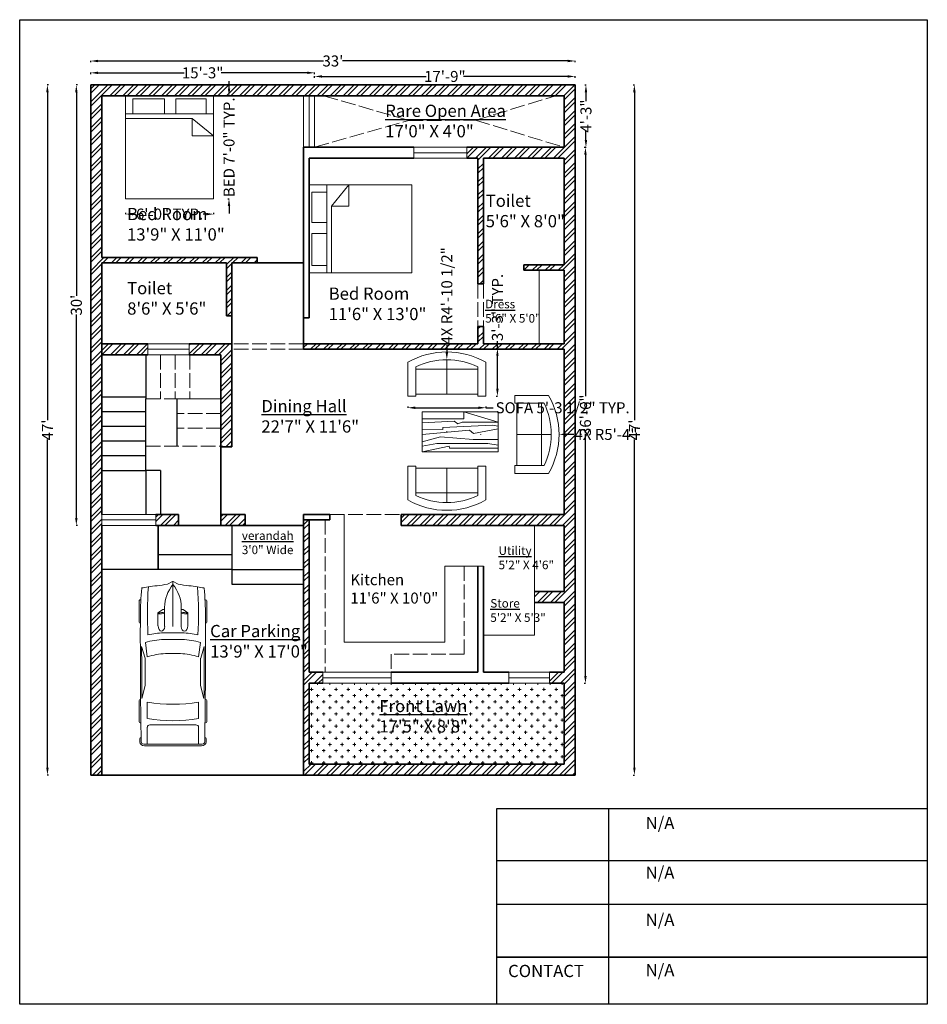
# Model space of a CAD drawing. Units: inches. Extents: x -42 to 700, y -732 to 72.
import ezdxf

# ---------------------------------------------------------------- set-up
doc = ezdxf.new("R2010")
doc.units = ezdxf.units.IN
doc.header["$MEASUREMENT"] = 0
doc.linetypes.add('ACAD_ISO02W100', pattern=[15, 12, -3])
for name, color, linetype, lineweight in [('A-ANNO-DIMS', 2, 'Continuous', 18), ('A-ANNO-TEXT', 7, 'Continuous', 18), ('A-ANNO-TTLB', 7, 'Continuous', 25), ('A-AREA-IDEN', 7, 'Continuous', 25), ('A-EQPM-VEHI', 8, 'Continuous', 18), ('A-FLOR-CASE', 8, 'Continuous', 18), ('A-FLOR-CASE-HIDN', 8, 'ACAD_ISO02W100', 13), ('A-FLOR-OPEN', 9, 'ACAD_ISO02W100', 13), ('A-FLOR-STRS', 6, 'Continuous', 25), ('A-FLOR-STRS-OVHD', 6, 'ACAD_ISO02W100', 18), ('A-FURN', 8, 'Continuous', 18), ('A-GLAZ', 5, 'Continuous', 18), ('A-WALL', 7, 'Continuous', 35), ('A-WALL-OVHD', 7, 'ACAD_ISO02W100', 18), ('A-WALL-PATT', 252, 'Continuous', 13), ('L-PLNT-PATT', 3, 'Continuous', 13)]:
    doc.layers.add(name, color=color, linetype=linetype, lineweight=lineweight)
doc.styles.get("Standard").update_dxf_attribs({"font": 'arial.ttf'})
doc.dimstyles.get("Standard").update_dxf_attribs({"dimtxt": 9, "dimasz": 6, "dimexe": 0.18, "dimexo": 0.0625, "dimgap": 0.09, "dimtad": 0, "dimdec": 0, "dimzin": 0, "dimdsep": 46, "dimlunit": 3, "dimtxsty": 'Standard', "dimcen": 0.09, "dimadec": 0, "dimazin": 0, "dimtfac": 1, "dimtdec": 0, "dimtofl": 0, "dimtmove": 0, "dimatfit": 3, "dimfxl": 1, "dimfxlon": 1, "dimtolj": 1, "dimtzin": 0, "dimarcsym": 0})

# ---------------------------------------------------------------- blocks, each defined once
blk = doc.blocks.new('A$C01575E38')
for p, q in [((0, 0), (0, 0.65)), ((0, 0), (0, 0.65)), ((0.75, 0.039), (0.75, 0.7)), ((0.75, 0.039), (0.75, 0.7)), ((1.5, 0.65), (1.5, 0)), ((1.5, 0.65), (1.5, 0)), ((0.15, 0), (0.15, 0.563)), ((0.15, 0), (0.15, 0.563)), ((0.15, 0.515), (1.35, 0.515)), ((0.15, 0.515), (1.35, 0.515)), ((1.35, 0), (1.35, 0.563)), ((1.35, 0), (1.35, 0.563)), ((0.15, 0), (0, 0)), ((0.15, 0), (0, 0)), ((0.15, 0.039), (1.35, 0.039)), ((0.15, 0.039), (1.35, 0.039)), ((1.5, 0), (1.35, 0)), ((1.5, 0), (1.35, 0))]:
    blk.add_line(p, q)
for centre, radius, start, end in [((0.75, -0.656), 1.506, 60.1372, 119.8628), ((0.75, -0.656), 1.506, 60.1372, 119.8628), ((0.75, -0.685), 1.385, 64.3208, 115.6792), ((0.75, -0.685), 1.385, 64.3208, 115.6792)]:
    blk.add_arc(centre, radius, start, end)
blk = doc.blocks.new('*U3')
for p, q in [((21.1, 37.4), (21.1, 36.8)), ((46.6, 38.9), (22.4, 38.9)), ((47.8, 37.4), (47.8, 37.4)), ((88, 31.9), (74.8, 35.9)), ((134.3, 35.6), (119.3, 31.8)), ((135.5, 37.1), (135.5, 37.4)), ((136.7, 38.9), (160.9, 38.9)), ((162.1, 37.4), (162.1, 36.8)), ((70, 31.5), (86.4, 29.4)), ((138.4, 29.4), (157.2, 29.4)), ((164.5, 26.4), (164.5, -26.4)), ((186.5, 29.4), (167, 29.4)), ((186.5, -33.5), (186.5, 33.5)), ((188.4, -32.8), (188.4, 32.8)), ((32.3, 11.6), (36.1, 17.2)), ((36.1, 17.2), (50.9, 17.2)), ((3.3, 6.1), (0.1, 0.4)), ((29.8, 9.5), (51.7, 9.5)), ((32.1, 9.5), (32.1, 11.2)), ((58.9, -10.8), (58.9, 10.8)), ((66.6, -10.5), (66.6, 10.5)), ((82.7, 8.5), (82.7, -8.5)), ((186.5, -10.5), (186.5, 10.5)), ((0, 0), (51.7, 0)), ((0.1, -0.4), (3.3, -6.1)), ((29.8, -9.5), (51.7, -9.5)), ((32.1, -9.5), (32.1, -11.2)), ((32.3, -11.6), (36.1, -17.2)), ((36.1, -17.2), (50.9, -17.2)), ((86.4, -29.4), (70, -31.5)), ((88, -31.9), (74.8, -35.9)), ((134.3, -35.6), (119.3, -31.8)), ((157.2, -29.4), (138.4, -29.4)), ((167, -29.4), (186.5, -29.4)), ((21.1, -37.4), (21.1, -36.8)), ((46.6, -38.9), (22.4, -38.9)), ((47.8, -37.4), (47.8, -37.4)), ((135.5, -37.1), (135.5, -37.4)), ((136.7, -38.9), (160.9, -38.9)), ((162.1, -37.4), (162.1, -36.8))]:
    blk.add_line(p, q)
for centre, major_axis, ratio, start_param, end_param in [((266, -27.5), (0, 313.3), 0.842304, 1.367076, 1.39176), ((41.2, -490.9), (0, 528.2), 0.842304, 0.00281, 0.075598), ((22.4, 37.4), (0, -1.48), 0.842304, 3.141593, 4.712389), ((64.5, -10555.6), (0, 10593), 0.842304, -0.013397, 0.002797), ((46.6, 37.4), (0, 1.48), 0.842304, -1.570796, 0), ((64.5, -10555.6), (0, -10591.5), 0.842304, 3.133765, 3.140441), ((136.7, 37.4), (0, -1.48), 0.842304, 3.141593, 4.712389), ((160.9, 37.4), (0, 1.48), 0.842304, -1.570796, 0), ((180.6, 35.8), (0, 2.22), 0.842304, -0.013017, 1.249894), ((64.5, -10556.4), (0, 10595.3), 0.842304, -0.013397, -0.013017), ((184, 32.8), (0, -5.25), 0.842304, 1.570796, 3.128196), ((184, 33.5), (0, -2.96), 0.842304, 1.570796, 3.128196), ((259.2, -27.5), (0, -305.3), 0.842304, 4.528606, 4.561838), ((37.5, -594), (0, -623.3), 0.842304, 3.096046, 3.200911), ((134.4, 5.4), (0, -89.8), 0.842304, 4.449482, 4.652344), ((135.3, 5.4), (0, 81.8), 0.842304, 1.245306, 1.50788), ((149.6, 2.8), (0, -79.6), 0.842304, 4.372215, 4.640744), ((95.8, -3666.4), (0, -3698.2), 0.842304, 3.134049, 3.144098), ((17.1, 0), (0, 147), 0.842304, 4.511394, 4.913384), ((35.9, 0), (0, 147), 0.842304, 4.511394, 4.913384), ((167, 26.4), (0, 2.96), 0.842304, 0, 1.570796), ((-204.5, 52.4), (0, -251), 0.842304, 1.385369, 1.434372), ((32.7, 11.2), (0, 0.74), 0.842304, 0.879714, 1.570796), ((13, 17), (0, 27.4), 0.842304, 4.435146, 4.718221), ((14.2, 17), (0, 27.4), 0.842304, 4.435146, 4.718221), ((50.8, 13.3), (6.34, -0.36), 0.603834, -1.395552, 1.581315), ((0.6, 0), (0, -0.74), 0.842304, 4.131459, 5.293319), ((29.8, -46.7), (0, 56.2), 0.842304, 0, 0.590319), ((-204.5, -52.4), (0, 251), 0.842304, -1.434372, -1.385369), ((29.8, 46.7), (0, 56.2), 0.842304, 2.551274, 3.141593), ((32.7, -11.2), (0, -0.74), 0.842304, 4.712389, 5.403472), ((13, -17), (0, -27.4), 0.842304, 1.564964, 1.848039), ((14.2, -17), (0, -27.4), 0.842304, 1.564964, 1.848039), ((134.4, -5.4), (0, -89.8), 0.842304, -1.510751, -1.307889), ((135.3, -5.4), (0, -81.8), 0.842304, -1.50788, -1.245306), ((149.6, -2.8), (0, -79.6), 0.842304, -1.499151, -1.230623), ((259.2, 27.5), (0, 305.3), 0.842304, 1.721348, 1.754579), ((266, 27.5), (0, 313.3), 0.842304, 1.749832, 1.774517), ((37.5, 594), (0, -623.3), 0.842304, -0.059319, 0.045547), ((95.8, 3666.4), (0, -3698.2), 0.842304, -0.002505, 0.007544), ((167, -26.4), (0, -2.96), 0.842304, 4.712389, 6.283185), ((184, -32.8), (0, -5.25), 0.842304, 0.013397, 1.570796), ((184, -33.5), (0, 2.96), 0.842304, 3.15499, 4.712389), ((41.2, 490.9), (0, -528.2), 0.842304, -0.075598, -0.00281), ((22.4, -37.4), (0, 1.48), 0.842304, 1.570796, 3.141593), ((64.5, 10555.6), (0, 10593), 0.842304, 3.138796, 3.15499), ((46.6, -37.4), (0, -1.48), 0.842304, 0, 1.570796), ((64.5, 10555.6), (0, -10591.5), 0.842304, 0.001152, 0.007828), ((136.7, -37.4), (0, -1.48), 0.842304, -1.570796, 0), ((160.9, -37.4), (0, 1.48), 0.842304, 3.141593, 4.712389), ((180.6, -35.8), (0, -2.22), 0.842304, -1.249894, 0.013017), ((64.5, 10556.4), (0, 10595.3), 0.842304, 3.15461, 3.15499)]:
    blk.add_ellipse(centre, major_axis=major_axis, ratio=ratio, start_param=start_param, end_param=end_param)
at = {"extrusion": (0, 0, -1)}
blk.add_ellipse((50.8, -13.3), major_axis=(6.34, 0.36), ratio=0.603834, start_param=-1.395552, end_param=1.581315, dxfattribs=at)
blk = doc.blocks.new('*D4')
at = {"layer": 'A-ANNO-DIMS', "color": 0, "lineweight": -2, "transparency": 16777216}
for p, q in [((15.72, 27.92), (15.72, 29.1)), ((21.72, 28.92), (92.09, 28.92)), ((192.72, 28.92), (122.34, 28.92)), ((198.72, 27.92), (198.72, 29.1))]:
    blk.add_line(p, q, dxfattribs=at)
at = {"layer": 'A-ANNO-DIMS', "color": 0, "transparency": 16777216}
for points in [[(21.72, 29.92), (21.72, 27.92), (15.72, 28.92)], [(192.72, 29.92), (192.72, 27.92), (198.72, 28.92)]]:
    blk.add_solid(points, dxfattribs=at)
at = {"layer": 'Defpoints', "color": 0, "transparency": 16777216}
for p in [(198.72, 28.92), (15.72, 19.05), (198.72, 19.05)]:
    blk.add_point(p, dxfattribs=at)
at = {"layer": 'A-ANNO-DIMS', "color": 0, "transparency": 16777216, "insert": (107.22, 28.92), "char_height": 9, "attachment_point": 5}
blk.add_mtext('\\A1;15\'-3"', dxfattribs=at)
blk = doc.blocks.new('*D5')
at = {"layer": 'A-ANNO-DIMS', "color": 0, "lineweight": -2, "transparency": 16777216}
for p, q in [((15.72, 37.59), (15.72, 38.77)), ((21.72, 38.59), (205.99, 38.59)), ((405.72, 38.59), (221.44, 38.59)), ((411.72, 37.59), (411.72, 38.77))]:
    blk.add_line(p, q, dxfattribs=at)
at = {"layer": 'A-ANNO-DIMS', "color": 0, "transparency": 16777216}
for points in [[(21.72, 39.59), (21.72, 37.59), (15.72, 38.59)], [(405.72, 39.59), (405.72, 37.59), (411.72, 38.59)]]:
    blk.add_solid(points, dxfattribs=at)
at = {"layer": 'Defpoints', "color": 0, "transparency": 16777216}
for p in [(411.72, 38.59), (15.72, 19.05), (411.72, 19.05)]:
    blk.add_point(p, dxfattribs=at)
at = {"layer": 'A-ANNO-DIMS', "color": 0, "transparency": 16777216, "insert": (213.72, 38.59), "char_height": 9, "attachment_point": 5}
blk.add_mtext("\\A1;33'", dxfattribs=at)
blk = doc.blocks.new('*D6')
at = {"layer": 'A-ANNO-DIMS', "color": 0, "lineweight": -2, "transparency": 16777216}
for p, q in [((198.72, 24.95), (198.72, 26.13)), ((204.72, 25.95), (290.09, 25.95)), ((405.72, 25.95), (320.34, 25.95)), ((411.72, 24.95), (411.72, 26.13))]:
    blk.add_line(p, q, dxfattribs=at)
at = {"layer": 'A-ANNO-DIMS', "color": 0, "transparency": 16777216}
for points in [[(204.72, 26.95), (204.72, 24.95), (198.72, 25.95)], [(405.72, 26.95), (405.72, 24.95), (411.72, 25.95)]]:
    blk.add_solid(points, dxfattribs=at)
at = {"layer": 'Defpoints', "color": 0, "transparency": 16777216}
for p in [(411.72, 25.95), (198.72, 19.05), (411.72, 19.05)]:
    blk.add_point(p, dxfattribs=at)
at = {"layer": 'A-ANNO-DIMS', "color": 0, "transparency": 16777216, "insert": (305.22, 25.95), "char_height": 9, "attachment_point": 5}
blk.add_mtext('\\A1;17\'-9"', dxfattribs=at)
blk = doc.blocks.new('*D7')
at = {"layer": 'A-ANNO-DIMS', "color": 0, "lineweight": -2, "transparency": 16777216}
for p, q in [((419.57, 19.05), (420.75, 19.05)), ((420.57, 13.05), (420.57, 5.78)), ((420.57, -25.95), (420.57, -18.68)), ((419.57, -31.95), (420.75, -31.95))]:
    blk.add_line(p, q, dxfattribs=at)
at = {"layer": 'A-ANNO-DIMS', "color": 0, "transparency": 16777216}
for points in [[(419.57, 13.05), (421.57, 13.05), (420.57, 19.05)], [(419.57, -25.95), (421.57, -25.95), (420.57, -31.95)]]:
    blk.add_solid(points, dxfattribs=at)
at = {"layer": 'Defpoints', "color": 0, "transparency": 16777216}
for p in [(411.72, 19.05), (410.47, -31.95), (420.57, -31.95)]:
    blk.add_point(p, dxfattribs=at)
at = {"layer": 'A-ANNO-DIMS', "color": 0, "transparency": 16777216, "insert": (420.57, -6.45), "char_height": 9, "attachment_point": 5, "rotation": 90}
blk.add_mtext('\\A1;4\'-3"', dxfattribs=at)
blk = doc.blocks.new('*D8')
at = {"layer": 'A-ANNO-DIMS', "color": 0, "lineweight": -2, "transparency": 16777216}
for p, q in [((459.16, 19.05), (460.34, 19.05)), ((460.16, 13.05), (460.16, -255.04)), ((460.16, -538.95), (460.16, -270.86)), ((459.16, -544.95), (460.34, -544.95))]:
    blk.add_line(p, q, dxfattribs=at)
at = {"layer": 'A-ANNO-DIMS', "color": 0, "transparency": 16777216}
for points in [[(459.16, 13.05), (461.16, 13.05), (460.16, 19.05)], [(459.16, -538.95), (461.16, -538.95), (460.16, -544.95)]]:
    blk.add_solid(points, dxfattribs=at)
at = {"layer": 'Defpoints', "color": 0, "transparency": 16777216}
for p in [(411.72, 19.05), (411.72, -544.95), (460.16, -544.95)]:
    blk.add_point(p, dxfattribs=at)
at = {"layer": 'A-ANNO-DIMS', "color": 0, "transparency": 16777216, "insert": (460.16, -262.95), "char_height": 9, "attachment_point": 5, "rotation": 90}
blk.add_mtext("\\A1;47'", dxfattribs=at)
blk = doc.blocks.new('*D9')
at = {"layer": 'A-ANNO-DIMS', "color": 0, "lineweight": -2, "transparency": 16777216}
for p, q in [((419.16, -31.95), (420.34, -31.95)), ((420.16, -37.95), (420.16, -235.4)), ((420.16, -463.95), (420.16, -266.49)), ((419.16, -469.95), (420.34, -469.95))]:
    blk.add_line(p, q, dxfattribs=at)
at = {"layer": 'A-ANNO-DIMS', "color": 0, "transparency": 16777216}
for points in [[(419.16, -37.95), (421.16, -37.95), (420.16, -31.95)], [(419.16, -463.95), (421.16, -463.95), (420.16, -469.95)]]:
    blk.add_solid(points, dxfattribs=at)
at = {"layer": 'Defpoints', "color": 0, "transparency": 16777216}
for p in [(402.72, -31.95), (402.72, -469.95), (420.16, -469.95)]:
    blk.add_point(p, dxfattribs=at)
at = {"layer": 'A-ANNO-DIMS', "color": 0, "transparency": 16777216, "insert": (420.16, -250.95), "char_height": 9, "attachment_point": 5, "rotation": 90}
blk.add_mtext('\\A1;36\'-6"', dxfattribs=at)
blk = doc.blocks.new('*D10')
at = {"layer": 'A-ANNO-DIMS', "color": 0, "lineweight": -2, "transparency": 16777216}
for p, q in [((-18.65, 19.05), (-19.83, 19.05)), ((-19.65, 13.05), (-19.65, -255.04)), ((-19.65, -538.95), (-19.65, -270.86)), ((-18.65, -544.95), (-19.83, -544.95))]:
    blk.add_line(p, q, dxfattribs=at)
at = {"layer": 'A-ANNO-DIMS', "color": 0, "transparency": 16777216}
for points in [[(-20.65, 13.05), (-18.65, 13.05), (-19.65, 19.05)], [(-20.65, -538.95), (-18.65, -538.95), (-19.65, -544.95)]]:
    blk.add_solid(points, dxfattribs=at)
at = {"layer": 'Defpoints', "color": 0, "transparency": 16777216}
for p in [(15.72, 19.05), (-19.65, -544.95), (15.72, -544.95)]:
    blk.add_point(p, dxfattribs=at)
at = {"layer": 'A-ANNO-DIMS', "color": 0, "transparency": 16777216, "insert": (-19.65, -262.95), "char_height": 9, "attachment_point": 5, "rotation": 90}
blk.add_mtext("\\A1;47'", dxfattribs=at)
blk = doc.blocks.new('*D11')
at = {"layer": 'A-ANNO-DIMS', "color": 0, "lineweight": -2, "transparency": 16777216}
for p, q in [((4.98, 19.05), (3.8, 19.05)), ((3.98, 13.05), (3.98, -153.22)), ((3.98, -334.95), (3.98, -168.67)), ((4.98, -340.95), (3.8, -340.95))]:
    blk.add_line(p, q, dxfattribs=at)
at = {"layer": 'A-ANNO-DIMS', "color": 0, "transparency": 16777216}
for points in [[(2.98, 13.05), (4.98, 13.05), (3.98, 19.05)], [(2.98, -334.95), (4.98, -334.95), (3.98, -340.95)]]:
    blk.add_solid(points, dxfattribs=at)
at = {"layer": 'Defpoints', "color": 0, "transparency": 16777216}
for p in [(15.72, 19.05), (3.98, -340.95), (24.72, -340.95)]:
    blk.add_point(p, dxfattribs=at)
at = {"layer": 'A-ANNO-DIMS', "color": 0, "transparency": 16777216, "insert": (3.98, -160.95), "char_height": 9, "attachment_point": 5, "rotation": 90}
blk.add_mtext("\\A1;30'", dxfattribs=at)
blk = doc.blocks.new('BED-72X84')
for p, q in [((0, 84), (0, 0)), ((72, 0), (72, 84)), ((0, 69.48), (72, 69.48)), ((0, 65.63), (54.47, 65.63)), ((54.47, 65.63), (54.47, 51.42)), ((72, 51.42), (54.47, 65.63)), ((54.47, 51.42), (72, 51.42)), ((0, 0), (72, 0))]:
    blk.add_line(p, q)
for points in [[(6.02, 81.67), (31.99, 81.67), (31.99, 69.48), (6.02, 69.48)], [(65.98, 81.67), (41.03, 81.67), (41.03, 69.48), (65.98, 69.48)]]:
    blk.add_lwpolyline(points, close=True)
blk = doc.blocks.new('*D13')
at = {"layer": 'A-ANNO-DIMS', "color": 0, "lineweight": -2, "transparency": 16777216}
for p, q in [((128.79, 16.05), (128.79, 22.05)), ((127.79, 10.05), (128.97, 10.05)), ((127.79, -73.95), (128.97, -73.95)), ((128.79, -79.95), (128.79, -85.95))]:
    blk.add_line(p, q, dxfattribs=at)
at = {"layer": 'A-ANNO-DIMS', "color": 0, "transparency": 16777216}
for points in [[(127.79, 16.05), (129.79, 16.05), (128.79, 10.05)], [(127.79, -79.95), (129.79, -79.95), (128.79, -73.95)]]:
    blk.add_solid(points, dxfattribs=at)
at = {"layer": 'Defpoints', "color": 0, "transparency": 16777216}
for p in [(116.19, 10.05), (128.79, 10.05), (116.19, -73.95)]:
    blk.add_point(p, dxfattribs=at)
at = {"layer": 'A-ANNO-DIMS', "color": 0, "transparency": 16777216, "insert": (128.79, -31.95), "char_height": 9, "attachment_point": 5, "rotation": 90}
blk.add_mtext('\\A1;BED 7\'-0" TYP.', dxfattribs=at)
blk = doc.blocks.new('*D14')
at = {"layer": 'A-ANNO-DIMS', "color": 0, "lineweight": -2, "transparency": 16777216}
for p, q in [((44.19, -85.55), (44.19, -86.73)), ((50.19, -86.55), (52.65, -86.55)), ((110.19, -86.55), (107.74, -86.55)), ((116.19, -85.55), (116.19, -86.73))]:
    blk.add_line(p, q, dxfattribs=at)
at = {"layer": 'A-ANNO-DIMS', "color": 0, "transparency": 16777216}
for points in [[(50.19, -85.55), (50.19, -87.55), (44.19, -86.55)], [(110.19, -85.55), (110.19, -87.55), (116.19, -86.55)]]:
    blk.add_solid(points, dxfattribs=at)
at = {"layer": 'Defpoints', "color": 0, "transparency": 16777216}
for p in [(44.19, -73.95), (116.19, -73.95), (116.19, -86.55)]:
    blk.add_point(p, dxfattribs=at)
at = {"layer": 'A-ANNO-DIMS', "color": 0, "transparency": 16777216, "insert": (80.19, -86.55), "char_height": 9, "attachment_point": 5}
blk.add_mtext('\\A1;6\'-0" TYP.', dxfattribs=at)
blk = doc.blocks.new('*D15')
at = {"layer": 'A-ANNO-DIMS', "color": 0, "lineweight": -2, "transparency": 16777216}
for p, q in [((275.02, -243.8), (275.02, -244.98)), ((281.02, -244.8), (332.66, -244.8)), ((338.66, -243.8), (338.66, -244.98)), ((338.66, -244.8), (344.66, -244.8))]:
    blk.add_line(p, q, dxfattribs=at)
at = {"layer": 'A-ANNO-DIMS', "color": 0, "transparency": 16777216}
for points in [[(281.02, -243.8), (281.02, -245.8), (275.02, -244.8)], [(332.66, -243.8), (332.66, -245.8), (338.66, -244.8)]]:
    blk.add_solid(points, dxfattribs=at)
at = {"layer": 'Defpoints', "color": 0, "transparency": 16777216}
for p in [(275.02, -235.25), (338.66, -235.25), (338.66, -244.8)]:
    blk.add_point(p, dxfattribs=at)
at = {"layer": 'A-ANNO-DIMS', "color": 0, "transparency": 16777216, "insert": (401.51, -244.8), "char_height": 9, "attachment_point": 5}
blk.add_mtext('\\A1;SOFA 5\'-3 1/2" TYP.', dxfattribs=at)
blk = doc.blocks.new('*D16')
at = {"layer": 'A-ANNO-DIMS', "color": 0, "lineweight": -2, "transparency": 16777216}
for p, q in [((348.2, -196.36), (348.2, -190.36)), ((347.2, -196.36), (348.38, -196.36)), ((348.2, -229.25), (348.2, -202.36)), ((347.2, -235.25), (348.38, -235.25))]:
    blk.add_line(p, q, dxfattribs=at)
at = {"layer": 'A-ANNO-DIMS', "color": 0, "transparency": 16777216}
for points in [[(347.2, -202.36), (349.2, -202.36), (348.2, -196.36)], [(347.2, -229.25), (349.2, -229.25), (348.2, -235.25)]]:
    blk.add_solid(points, dxfattribs=at)
at = {"layer": 'Defpoints', "color": 0, "transparency": 16777216}
for p in [(338.66, -196.36), (348.2, -196.36), (338.66, -235.25)]:
    blk.add_point(p, dxfattribs=at)
at = {"layer": 'A-ANNO-DIMS', "color": 0, "transparency": 16777216, "insert": (348.2, -162.85), "char_height": 9, "attachment_point": 5, "rotation": 90}
blk.add_mtext('\\A1;3\'-3" TYP.', dxfattribs=at)
blk = doc.blocks.new('*D17')
at = {"layer": 'A-ANNO-DIMS', "color": 0, "lineweight": -2, "transparency": 16777216}
for p, q in [((334.57, -266.59), (334.75, -266.59)), ((334.66, -266.68), (334.66, -266.5)), ((410.69, -266.59), (404.56, -266.59))]:
    blk.add_line(p, q, dxfattribs=at)
at = {"layer": 'A-ANNO-DIMS', "color": 0, "transparency": 16777216}
blk.add_solid([(404.56, -265.58), (404.56, -267.58), (398.56, -266.59)], dxfattribs=at)
at = {"layer": 'Defpoints', "color": 0, "transparency": 16777216}
for p in [(334.66, -266.59), (398.56, -266.59)]:
    blk.add_point(p, dxfattribs=at)
at = {"layer": 'A-ANNO-DIMS', "color": 0, "transparency": 16777216, "insert": (436.9, -266.59), "char_height": 9, "attachment_point": 5, "rotation": 0.00021}
blk.add_mtext('\\A1;4X R5\'-4"', dxfattribs=at)
blk = doc.blocks.new('*D18')
at = {"layer": 'A-ANNO-DIMS', "color": 0, "lineweight": -2, "transparency": 16777216}
for p, q in [((306.84, -193.56), (306.84, -199.56)), ((306.75, -264.29), (306.93, -264.29)), ((306.84, -264.38), (306.84, -264.2))]:
    blk.add_line(p, q, dxfattribs=at)
at = {"layer": 'A-ANNO-DIMS', "color": 0, "transparency": 16777216}
blk.add_solid([(305.84, -199.56), (307.84, -199.56), (306.84, -205.56)], dxfattribs=at)
at = {"layer": 'Defpoints', "color": 0, "transparency": 16777216}
for p in [(306.84, -205.56), (306.84, -264.29)]:
    blk.add_point(p, dxfattribs=at)
at = {"layer": 'A-ANNO-DIMS', "color": 0, "transparency": 16777216, "insert": (306.84, -153.36), "char_height": 9, "attachment_point": 5, "rotation": 89.99984}
blk.add_mtext('\\A1;4X R4\'-10 1/2"', dxfattribs=at)

msp = doc.modelspace()

# ---------------------------------------------------------------- hatches: boundary and pattern name
at = {"layer": 'A-WALL-PATT'}
h = msp.add_hatch(dxfattribs=at)
h.set_pattern_fill('ANSI32', color=256, scale=20)
h.paths.add_polyline_path([(402.72, 10.05), (402.72, -31.95), (323.2, -31.95), (323.2, -40.95), (332.22, -40.95), (332.22, -143.52), (336.72, -143.52), (336.72, -40.95), (402.72, -40.95), (402.72, -127.95), (369.72, -127.95), (369.72, -132.45), (402.72, -132.45), (402.72, -192.45), (336.72, -192.45), (336.72, -178.3), (332.22, -178.3), (332.22, -192.45), (189.72, -192.45), (189.72, -196.95), (194.22, -196.95), (402.72, -196.95), (402.72, -331.95), (269.49, -331.95), (269.49, -340.95), (402.72, -340.95), (402.72, -394.95), (378.4, -394.95), (378.4, -403.95), (402.72, -403.95), (402.72, -460.95), (390.78, -460.95), (390.78, -469.95), (402.72, -469.95), (402.72, -535.95), (194.22, -535.95), (194.22, -469.95), (205.4, -469.95), (205.4, -460.95), (194.22, -460.95), (194.22, -336.45), (189.72, -336.45), (189.72, -544.95), (411.72, -544.95), (411.72, 10.05), (411.72, 19.05), (15.72, 19.05), (15.72, -544.95), (24.72, -544.95), (24.72, -340.95), (24.72, -331.95), (24.72, -126.45), (126.72, -126.45), (126.72, -169.65), (131.22, -169.65), (131.22, -126.45), (151.89, -126.45), (151.89, -121.95), (131.22, -121.95), (24.72, -121.95), (24.72, 10.05)])
h.paths.add_polyline_path([(109.33, -454.62), (193.28, -454.62), (193.28, -417.31), (109.33, -417.31)], flags=25)
h = msp.add_hatch(dxfattribs=at)
h.set_pattern_fill('ANSI32', color=256, scale=20)
h.paths.add_polyline_path([(87.53, -331.95), (68.85, -331.95), (68.85, -340.95), (87.53, -340.95)])
h.paths.add_polyline_path([(142.09, -331.95), (131.22, -331.95), (122.22, -331.95), (122.22, -340.95), (142.09, -340.95)])
h.paths.add_polyline_path([(62.44, -192.45), (24.72, -192.45), (24.72, -201.45), (62.44, -201.45)])
h.paths.add_polyline_path([(131.22, -192.45), (96.25, -192.45), (96.25, -201.45), (122.22, -201.45), (122.22, -276.81), (131.22, -276.81)])
at = {"layer": 'L-PLNT-PATT'}
h = msp.add_hatch(dxfattribs=at)
h.set_pattern_fill('CROSS', color=256, scale=20)
h.paths.add_polyline_path([(402.72, -469.95), (390.78, -469.95), (357.5, -469.95), (261.21, -469.95), (205.4, -469.95), (194.22, -469.95), (194.22, -535.95), (402.72, -535.95)])

# ---------------------------------------------------------------- linework, layer by layer
at = {"layer": 'A-ANNO-TTLB'}
for p, q in [((439.07, -572.4), (439.07, -732.32)), ((347.75, -614.66), (699.63, -614.66)), ((347.75, -650.35), (699.63, -650.35)), ((347.75, -693.86), (699.63, -693.86)), ((699.63, -693.86), (347.75, -693.86))]:
    msp.add_line(p, q, dxfattribs=at)
for points in [[(-42.33, 72.33), (699.63, 72.33), (699.63, -732.32), (-42.33, -732.32)], [(347.75, -572.4), (699.63, -572.4), (699.63, -732.32), (347.75, -732.32)]]:
    msp.add_lwpolyline(points, close=True, dxfattribs=at)
at = {"layer": 'A-FLOR-CASE'}
for p, q in [((382.33, -132.45), (382.33, -192.45)), ((211.27, -331.95), (222.92, -331.95)), ((222.92, -331.95), (222.92, -436.33)), ((378.4, -430.69), (378.4, -340.95)), ((305.15, -436.33), (305.15, -374.27)), ((305.15, -374.27), (336.72, -374.27)), ((336.72, -430.69), (378.4, -430.69)), ((222.92, -436.33), (305.15, -436.33))]:
    msp.add_line(p, q, dxfattribs=at)
at = {"layer": 'A-FLOR-CASE-HIDN'}
for p, q in [((207.45, -336.45), (207.45, -460.95)), ((320.93, -374.27), (320.93, -446.16)), ((320.93, -446.16), (261.21, -446.16)), ((261.21, -446.16), (261.21, -460.95))]:
    msp.add_line(p, q, dxfattribs=at)
at = {"layer": 'A-FLOR-OPEN'}
for p, q in [((206.14, 10.05), (275.55, -9.79)), ((330.29, -9.89), (395.75, 10.05)), ((198.72, -31.95), (275.55, -9.99)), ((275.55, -9.79), (330.29, -9.89)), ((275.55, -9.99), (330.29, -9.89)), ((330.29, -9.89), (402.72, -31.95))]:
    msp.add_line(p, q, dxfattribs=at)
at = {"layer": 'A-FLOR-STRS'}
for p, q in [((60.72, -201.45), (60.72, -237.45)), ((24.72, -235.95), (60.72, -235.95)), ((60.72, -247.95), (60.72, -237.45)), ((86.22, -237.45), (86.22, -276.32)), ((24.72, -247.95), (60.72, -247.95)), ((60.72, -295.95), (60.72, -247.95)), ((24.72, -259.95), (60.72, -259.95)), ((24.72, -271.95), (60.72, -271.95)), ((24.72, -283.95), (60.72, -283.95)), ((24.72, -295.95), (60.72, -295.95)), ((60.72, -295.95), (60.72, -331.95)), ((72.72, -295.95), (60.72, -295.95)), ((72.72, -295.95), (72.72, -331.95)), ((70.85, -376.95), (70.85, -340.95)), ((70.85, -340.95), (70.85, -376.95)), ((131.22, -340.95), (131.22, -388.95)), ((131.22, -364.95), (70.85, -364.95)), ((70.85, -376.95), (24.72, -376.95)), ((131.22, -376.95), (70.85, -376.95)), ((131.22, -376.95), (189.72, -376.95)), ((131.22, -388.95), (189.72, -388.95))]:
    msp.add_line(p, q, dxfattribs=at)
at = {"layer": 'A-FLOR-STRS-OVHD'}
for p, q in [((72.72, -201.45), (72.72, -237.45)), ((84.72, -201.45), (84.72, -237.45)), ((96.72, -201.45), (96.72, -237.45)), ((60.72, -237.45), (122.22, -237.45)), ((122.22, -237.45), (86.22, -237.45)), ((122.22, -249.45), (86.22, -249.45)), ((122.22, -261.45), (86.22, -261.45)), ((60.72, -276.32), (123.69, -276.32))]:
    msp.add_line(p, q, dxfattribs=at)
at = {"layer": 'A-FURN'}
for p, q in [((320.72, -253.78), (320.72, -248.18)), ((320.72, -248.18), (348.93, -256.62)), ((286.57, -253.78), (286.57, -253.78)), ((286.57, -253.78), (320.72, -253.78)), ((312.72, -255.86), (286.57, -257.04)), ((315.79, -257.9), (312.72, -255.86)), ((319.45, -256.62), (315.79, -257.9)), ((348.93, -256.62), (319.45, -256.62)), ((286.57, -262.38), (286.57, -262.38)), ((286.57, -262.38), (303.66, -262.46)), ((325.39, -263.09), (286.57, -266.63)), ((303.66, -260.81), (343.97, -259.08)), ((303.66, -262.46), (303.66, -260.81)), ((328.78, -265.76), (325.39, -263.09)), ((348.93, -262.07), (328.78, -265.76)), ((343.97, -259.08), (348.93, -259.95)), ((286.57, -266.63), (286.57, -272.66)), ((286.57, -272.66), (301.58, -268.51)), ((301.58, -268.51), (328.41, -270.77)), ((328.41, -270.77), (348.93, -270.77)), ((348.93, -270.77), (348.93, -275.3)), ((298.68, -273.92), (286.57, -276.18)), ((286.57, -276.18), (286.57, -280.83)), ((286.57, -280.83), (308.63, -276.18)), ((315.69, -273.92), (298.68, -273.92)), ((308.63, -276.18), (308.97, -277.79)), ((308.97, -277.79), (348.93, -277.79)), ((340.5, -273.92), (315.69, -273.92)), ((348.93, -275.3), (340.5, -273.92))]:
    msp.add_line(p, q, dxfattribs=at)
msp.add_lwpolyline([(286.57, -248.18), (348.93, -248.18), (348.93, -280.83), (286.57, -280.83)], close=True, dxfattribs=at)
at = {"layer": 'A-GLAZ'}
for p, q in [((189.72, -31.95), (189.72, 10.05)), ((194.22, -31.95), (194.22, 10.05)), ((198.72, -31.95), (198.72, 10.05)), ((279.88, -31.95), (279.88, -40.95)), ((279.88, -31.95), (323.2, -31.95)), ((323.2, -31.95), (323.2, -40.95)), ((279.88, -36.45), (323.2, -36.45)), ((323.2, -40.95), (279.88, -40.95)), ((62.44, -192.45), (62.44, -201.45)), ((62.44, -192.45), (96.25, -192.45)), ((96.25, -192.45), (96.25, -201.45)), ((96.25, -196.95), (62.44, -196.95)), ((96.25, -201.45), (62.44, -201.45)), ((24.72, -331.95), (24.72, -340.95)), ((68.85, -331.95), (24.72, -331.95)), ((24.72, -336.45), (68.85, -336.45)), ((68.85, -331.95), (68.85, -340.95)), ((68.85, -340.95), (24.72, -340.95)), ((205.4, -460.95), (205.4, -469.95)), ((205.4, -460.95), (261.21, -460.95)), ((205.4, -465.45), (261.21, -465.45)), ((261.21, -460.95), (261.21, -469.95)), ((357.5, -460.95), (357.5, -469.95)), ((357.5, -460.95), (390.78, -460.95)), ((390.78, -465.45), (357.5, -465.45)), ((390.78, -460.95), (390.78, -469.95)), ((205.4, -469.95), (261.21, -469.95)), ((390.78, -469.95), (357.5, -469.95))]:
    msp.add_line(p, q, dxfattribs=at)
at = {"layer": 'A-WALL'}
for p, q in [((15.72, 19.05), (411.72, 19.05)), ((15.72, 19.05), (15.72, -544.95)), ((411.72, 19.05), (411.72, -46.95)), ((24.72, 10.05), (402.72, 10.05)), ((24.72, 10.05), (24.72, -121.95)), ((402.72, 10.05), (402.72, -31.95)), ((402.72, 10.05), (402.72, -31.95)), ((411.72, 10.05), (411.72, -544.95)), ((189.72, -31.95), (189.72, -196.95)), ((198.72, -31.95), (189.72, -31.95)), ((198.72, -31.95), (279.88, -31.95)), ((323.2, -31.95), (402.72, -31.95)), ((194.22, -40.95), (194.22, -171.22)), ((194.22, -40.95), (279.88, -40.95)), ((323.2, -40.95), (332.22, -40.95)), ((332.22, -40.95), (332.22, -143.52)), ((336.72, -40.95), (336.72, -143.52)), ((336.72, -40.95), (402.72, -40.95)), ((402.72, -40.95), (402.72, -127.95)), ((24.72, -121.95), (131.22, -121.95)), ((24.72, -126.45), (24.72, -331.95)), ((24.72, -126.45), (126.72, -126.45)), ((126.72, -126.45), (126.72, -169.65)), ((131.22, -121.95), (151.89, -121.95)), ((131.22, -126.45), (131.22, -276.81)), ((131.22, -126.45), (189.72, -126.45)), ((151.89, -121.95), (151.89, -126.45)), ((369.72, -127.95), (402.72, -127.95)), ((369.72, -127.95), (369.72, -132.45)), ((369.72, -132.45), (402.72, -132.45)), ((402.72, -132.45), (402.72, -192.45)), ((332.22, -143.52), (336.72, -143.52)), ((126.72, -169.65), (131.22, -169.65)), ((189.72, -171.22), (194.22, -171.22)), ((332.22, -178.3), (336.72, -178.3)), ((332.22, -178.3), (332.22, -192.45)), ((336.72, -178.3), (336.72, -192.45)), ((24.72, -192.45), (62.44, -192.45)), ((96.25, -192.45), (131.22, -192.45)), ((189.72, -192.45), (332.22, -192.45)), ((336.72, -192.45), (402.72, -192.45)), ((189.72, -196.95), (194.22, -196.95)), ((194.22, -196.95), (402.72, -196.95)), ((402.72, -196.95), (402.72, -331.95)), ((24.72, -201.45), (62.44, -201.45)), ((96.25, -201.45), (122.22, -201.45)), ((122.22, -201.45), (122.22, -340.95)), ((122.22, -276.81), (131.22, -276.81)), ((68.85, -331.95), (87.53, -331.95)), ((87.53, -331.95), (87.53, -340.95)), ((122.22, -331.95), (131.22, -331.95)), ((131.22, -331.95), (142.09, -331.95)), ((142.09, -331.95), (142.09, -340.95)), ((189.72, -331.95), (189.72, -544.95)), ((189.72, -331.95), (211.27, -331.95)), ((189.72, -336.45), (211.27, -336.45)), ((194.22, -336.45), (194.22, -460.95)), ((211.27, -331.95), (211.27, -336.45)), ((269.49, -331.95), (269.49, -340.95)), ((269.49, -331.95), (402.72, -331.95)), ((24.72, -340.95), (24.72, -544.95)), ((68.85, -340.95), (189.72, -340.95)), ((269.49, -340.95), (402.72, -340.95)), ((402.72, -340.95), (402.72, -394.95)), ((332.22, -374.27), (332.22, -460.95)), ((336.72, -374.27), (336.72, -460.95)), ((378.4, -394.95), (402.72, -394.95)), ((378.4, -403.95), (402.72, -403.95)), ((402.72, -403.95), (402.72, -460.95)), ((194.22, -460.95), (205.4, -460.95)), ((261.21, -460.95), (332.22, -460.95)), ((336.72, -460.95), (357.5, -460.95)), ((390.78, -460.95), (402.72, -460.95)), ((194.22, -469.95), (205.4, -469.95)), ((194.22, -469.95), (194.22, -535.95)), ((261.21, -469.95), (357.5, -469.95)), ((390.78, -469.95), (402.72, -469.95)), ((402.72, -469.95), (402.72, -535.95)), ((402.72, -535.95), (194.22, -535.95)), ((411.72, -544.95), (15.72, -544.95))]:
    msp.add_line(p, q, dxfattribs=at)
at = {"layer": 'A-WALL-OVHD'}
for p, q in [((332.22, -143.52), (332.22, -178.3)), ((336.72, -143.52), (336.72, -178.3)), ((189.72, -192.45), (131.22, -192.45)), ((189.72, -196.95), (131.22, -196.95)), ((211.27, -331.95), (269.49, -331.95))]:
    msp.add_line(p, q, dxfattribs=at)

# ---------------------------------------------------------------- block references
at = {"layer": 'A-EQPM-VEHI', "xscale": 0.7127593615244909, "yscale": 0.7127593615244909, "zscale": 0.7127593615244909, "rotation": 270}
msp.add_blockref('*U3', (82.95, -386.69), dxfattribs=at)
at = {"layer": 'A-FURN'}
msp.add_blockref('BED-72X84', (44.19, -73.95), dxfattribs=at)
at = {"layer": 'A-FURN', "rotation": 90}
msp.add_blockref('BED-72X84', (278.22, -134.49), dxfattribs=at)
at = {"layer": 'A-FURN', "xscale": 42.42261542958558, "yscale": 42.42261542958558, "zscale": 42.42261542958558}
msp.add_blockref('A$C01575E38', (275.02, -235.25), dxfattribs=at)
at = {"layer": 'A-FURN', "yscale": 42.42261542958558, "zscale": 42.42261542958558}
for p, xscale, rotation in [((362.5, -234.77), 42.42261542958558, 270), ((275.02, -292.56), -42.42261542958558, 180)]:
    msp.add_blockref('A$C01575E38', p, dxfattribs=dict(at, xscale=xscale, rotation=rotation))

# ---------------------------------------------------------------- texts
at = {"layer": 'A-ANNO-TEXT', "char_height": 10, "attachment_point": 1}
for s, width, insert in [('\\pxt17;N/A', 225.2095, (469.38, -579.12)), ('N/A', 221.8625, (469.38, -619.7)), ('N/A', 202.399, (469.38, -658.19)), ('CONTACT', 93.1868, (356.93, -700.06)), ('N/A', 93.1868, (469.38, -699.37))]:
    msp.add_mtext_dynamic_manual_height_columns(s, width=width, gutter_width=1, heights=[0], dxfattribs=dict(at, insert=insert))
at = {"layer": 'A-AREA-IDEN', "attachment_point": 1}
for s, width, insert, char_height in [('{\\LRare Open Area\\P}17\'0" X 4\'0"', 115.0179, (256.53, 2.87), 10), ('Toilet\\P5\'6" X 8\'0"', 93.1868, (338.63, -70.63), 10), ('Bed Room\\P13\'9" X 11\'0"', 93.1868, (45.4, -81.48), 10), ('Toilet\\P8\'6" X 5\'6"', 93.1868, (45.54, -142.03), 10), ('Bed Room\\P11\'6" X 13\'0"', 93.1868, (210.27, -146.54), 10), ('{\\LDress\\P}5\'6" X 5\'0"', 93.1868, (338.19, -156.55), 7), ('{\\LDining Hall\\P}22\'7" X 11\'6"', 93.1868, (155.24, -238.44), 10), ('{\\Lverandah\\P}3\'0" Wide', 93.1868, (139.29, -345.77), 7), ('{\\LUtility\\P}5\'2" X 4\'6"', 93.1868, (349.14, -358.09), 7), ('Kitchen\\P11\'6" X 10\'0"', 93.1868, (227.99, -380.81), 9), ('{\\LStore\\P}5\'2" X 5\'3"', 93.1868, (342.4, -401.11), 7), ('{\\LCar Parking\\P}13\'9" X 17\'0"', 93.1868, (113.35, -422.28), 10), ('{\\LFront Lawn\\P}17\'5" X 8\'8"', 93.1868, (251.73, -483.52), 10)]:
    msp.add_mtext_dynamic_manual_height_columns(s, width=width, gutter_width=1, heights=[0], dxfattribs=dict(at, insert=insert, char_height=char_height))

# ---------------------------------------------------------------- dimensions: what is measured, and where the dimension line sits
at = {"layer": 'A-ANNO-DIMS'}
for base, p1, p2, picture, middle in [((411.72, 38.59), (15.72, 19.05), (411.72, 19.05), '*D5', (213.72, 38.59)), ((198.72, 28.92), (15.72, 19.05), (198.72, 19.05), '*D4', (107.22, 28.92)), ((411.72, 25.95), (198.72, 19.05), (411.72, 19.05), '*D6', (305.22, 25.95))]:
    dim = msp.add_linear_dim(base=base, p1=p1, p2=p2, dimstyle='Standard', override={"dimclrd": 0, "dimclre": 0, "dimclrt": 0}, dxfattribs=at)
    dim.commit()
    dim.dimension.update_dxf_attribs({"geometry": picture, "text_midpoint": middle})
for base, p1, p2, picture, middle in [((-19.65, -544.95), (15.72, 19.05), (15.72, -544.95), '*D10', (-19.65, -262.95)), ((3.98, -340.95), (15.72, 19.05), (24.72, -340.95), '*D11', (3.98, -160.95)), ((420.57, -31.95), (411.72, 19.05), (410.47, -31.95), '*D7', (420.57, -6.45)), ((460.16, -544.95), (411.72, 19.05), (411.72, -544.95), '*D8', (460.16, -262.95)), ((420.16, -469.95), (402.72, -31.95), (402.72, -469.95), '*D9', (420.16, -250.95))]:
    dim = msp.add_linear_dim(base=base, p1=p1, p2=p2, angle=90, dimstyle='Standard', override={"dimclrd": 0, "dimclre": 0, "dimclrt": 0}, dxfattribs=at)
    dim.commit()
    dim.dimension.update_dxf_attribs({"geometry": picture, "text_midpoint": middle})
for base, p1, p2, text, picture, middle in [((128.79, 10.05), (116.19, -73.95), (116.19, 10.05), 'BED <> TYP.', '*D13', (128.79, -31.95)), ((348.2, -196.36), (338.66, -235.25), (338.66, -196.36), '<> TYP.', '*D16', (348.2, -162.85))]:
    dim = msp.add_linear_dim(base=base, p1=p1, p2=p2, angle=90, text=text, dimstyle='Standard', override={"dimdec": 1, "dimlfac": 1, "dimrnd": 0, "dimzin": 1, "dimdsep": 46, "dimlunit": 4, "dimfrac": 2}, dxfattribs=at)
    dim.commit()
    dim.dimension.update_dxf_attribs({"geometry": picture, "text_midpoint": middle})
for base, p1, p2, text, picture, middle in [((116.19, -86.55), (44.19, -73.95), (116.19, -73.95), '<> TYP.', '*D14', (80.19, -86.55)), ((338.66, -244.8), (275.02, -235.25), (338.66, -235.25), 'SOFA <> TYP.', '*D15', (401.51, -244.8))]:
    dim = msp.add_linear_dim(base=base, p1=p1, p2=p2, text=text, dimstyle='Standard', override={"dimdec": 1, "dimlfac": 1, "dimrnd": 0, "dimzin": 1, "dimdsep": 46, "dimlunit": 4, "dimfrac": 2}, dxfattribs=at)
    dim.commit()
    dim.dimension.update_dxf_attribs({"geometry": picture, "text_midpoint": middle})
dim = msp.add_radius_dim(center=(306.84, -264.29), mpoint=(306.84, -205.56), text='4X <>', dimstyle='Standard', override={"dimdec": 1, "dimlfac": 1, "dimrnd": 0, "dimzin": 1, "dimdsep": 46, "dimlunit": 4, "dimfrac": 2}, dxfattribs=at)
dim.commit()
dim.dimension.update_dxf_attribs({"geometry": '*D18', "text_midpoint": (306.84, -153.36)})
dim = msp.add_radius_dim(center=(334.66, -266.59), mpoint=(398.56, -266.59), text='4X <>', dimstyle='Standard', override={"dimdec": 1, "dimlfac": 1, "dimrnd": 0, "dimzin": 1, "dimdsep": 46, "dimlunit": 4, "dimfrac": 2}, dxfattribs=at)
dim.commit()
dim.dimension.update_dxf_attribs({"geometry": '*D17', "text_midpoint": (436.9, -266.58), "dimtype": 164})

doc.saveas('drawing.dxf')
